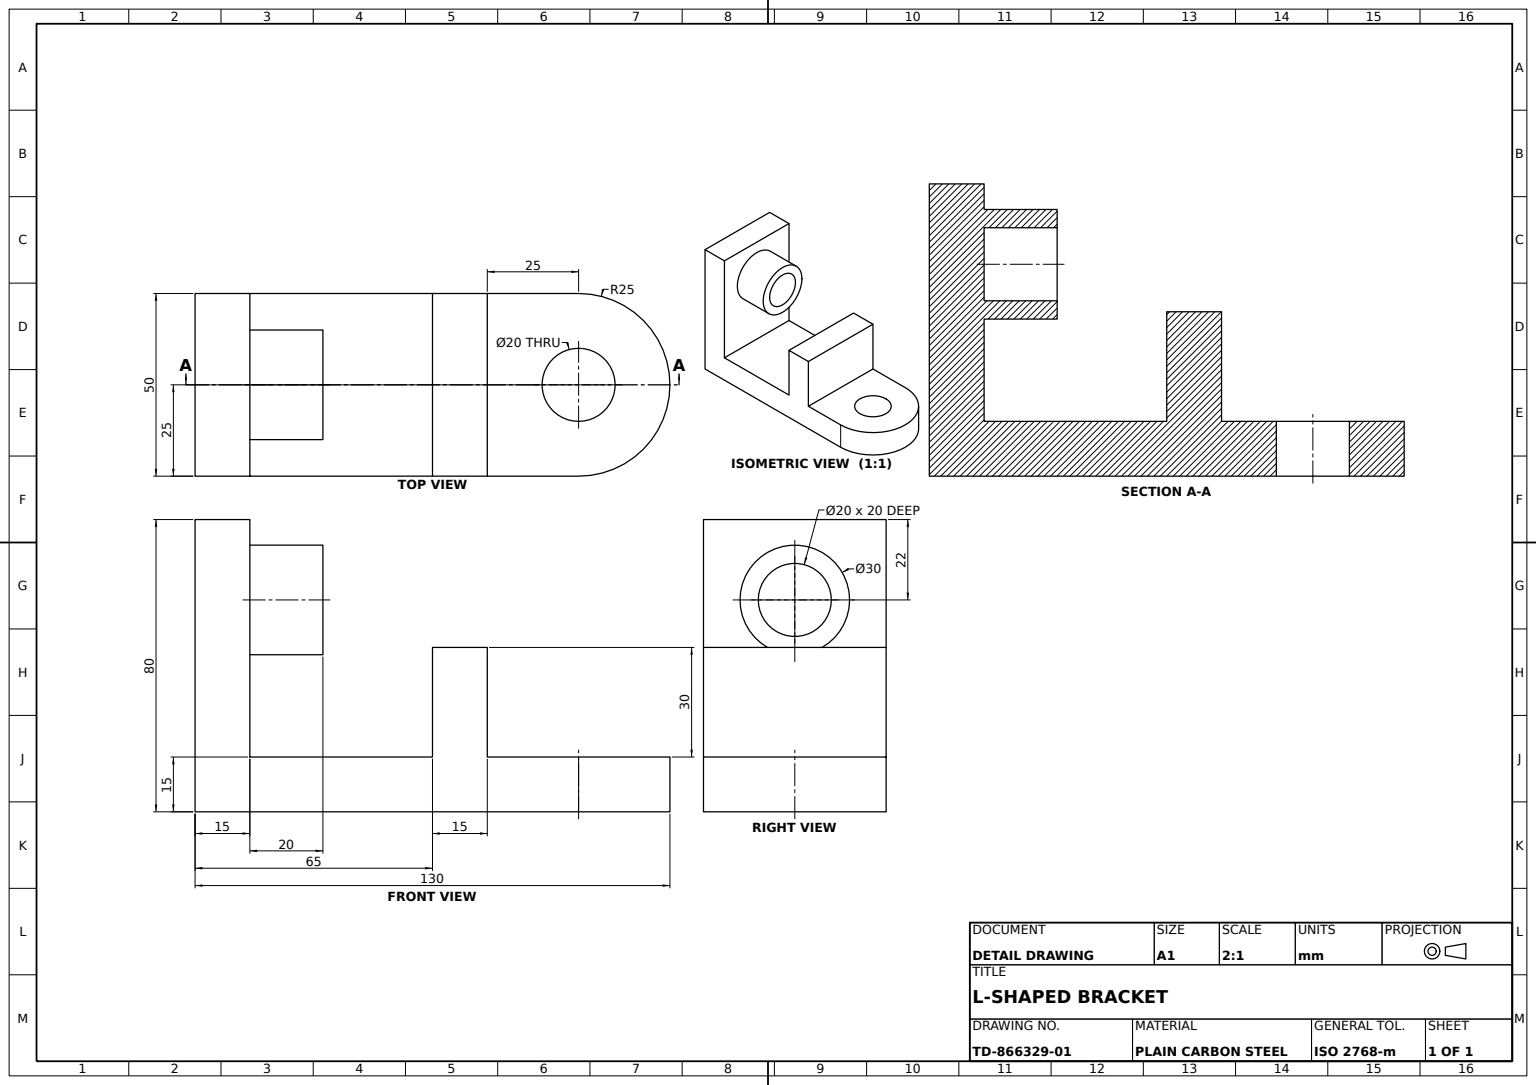
from build123d import *

# Parameters (mm, degrees)
BASE_PLATE_DEPTH      = 15
UPRIGHT_WALL_SKETCH_W = 15
UPRIGHT_WALL_SKETCH_H = 50
UPRIGHT_WALL_DEPTH    = 65
WALL_BOSS_SKETCH_R    = 15
WALL_BOSS_DEPTH       = 20
BOSS_BORE_SKETCH_R    = 10
BOSS_BORE_10_DEPTH    = 20
RAISED_BLOCK_SKETCH_W = 15
RAISED_BLOCK_SKETCH_H = 50
RAISED_BLOCK_DEPTH    = 30
LUG_HOLE_SKETCH_R     = 10
LUG_HOLE_DEPTH        = 15


with BuildPart() as part:
    # Base Plate Sketch → Base Plate (new body)
    with BuildSketch(Plane(origin=(0, 0, 0), x_dir=(1, 0, 0), z_dir=(0, 1, 0))):
        with BuildLine():
            Line((-65, -25), (40, -25))
            ThreePointArc((40, -25), (65, 0), (40, 25))
            Line((40, 25), (-65, 25))
            Line((-65, 25), (-65, -25))
        make_face()
    extrude(amount=BASE_PLATE_DEPTH)

    # Upright Wall Sketch → Upright Wall (add)
    with BuildSketch(Plane(origin=(0, 15, 0), x_dir=(1, 0, 0), z_dir=(0, 1, 0))):
        with Locations((-57.5, 0)):
            Rectangle(UPRIGHT_WALL_SKETCH_W, UPRIGHT_WALL_SKETCH_H)
    extrude(amount=UPRIGHT_WALL_DEPTH)

    # Wall Boss Sketch → Wall Boss (add)
    with BuildSketch(Plane(origin=(-50, 0, 0), x_dir=(0, 0, -1), z_dir=(1, 0, 0))):
        with Locations(Location((0, 58, 0), (0, 0, 180))):
            Circle(WALL_BOSS_SKETCH_R)
    extrude(amount=WALL_BOSS_DEPTH)

    # Boss Bore Sketch → Boss Bore Ø10 (cut)
    with BuildSketch(Plane(origin=(-30, 0, 0), x_dir=(0, 0, -1), z_dir=(1, 0, 0))):
        with Locations((0, 58)):
            Circle(BOSS_BORE_SKETCH_R)
    extrude(amount=-BOSS_BORE_10_DEPTH, mode=Mode.SUBTRACT)

    # Raised Block Sketch → Raised Block (add)
    with BuildSketch(Plane(origin=(0, 15, 0), x_dir=(1, 0, 0), z_dir=(0, 1, 0))):
        with Locations((7.5, 0)):
            Rectangle(RAISED_BLOCK_SKETCH_W, RAISED_BLOCK_SKETCH_H)
    extrude(amount=RAISED_BLOCK_DEPTH)

    # Lug Hole Sketch → Lug Hole (cut)
    with BuildSketch(Plane(origin=(0, 15, 0), x_dir=(1, 0, 0), z_dir=(0, 1, 0))):
        with Locations(Location((40, 0, 0), (0, 0, 270))):
            Circle(LUG_HOLE_SKETCH_R)
    extrude(amount=-LUG_HOLE_DEPTH, mode=Mode.SUBTRACT)


solid = part.part
